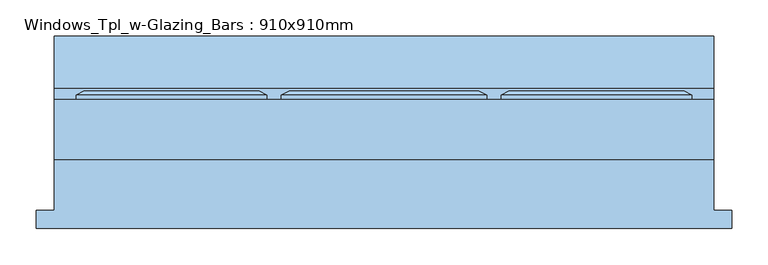
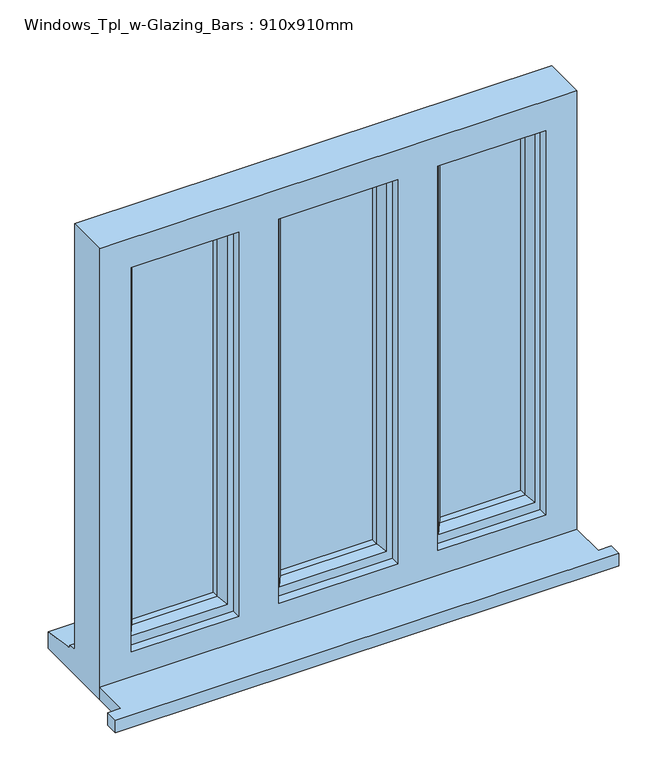
"""IFC4 building model written with IfcOpenShell, lengths in millimetres: window geometry, Windows_Tpl_w-Glazing_Bars : 910x910mm."""

from ifc_helpers import new_model, si_unit, frame, origin, place, context, project, spatial, polyline, outline, extrude, faceted_brep, source, transform, mapped, element, save


def windows_tpl_w_glazing_bars_910x910mm_9d987a72(model_context):
    return source(origin(), model_context, "Body", "SolidModel", [
        extrude(outline(polyline([(-716.6666667, -118.1434322), (-716.6666667, -93.1434322), (-691.6666667, -93.1434322), (-691.6666667, -22.9434322), (218.3333333, -22.9434322), (218.3333333, -93.1434322), (243.3333333, -93.1434322), (243.3333333, -118.1434322), (-716.6666667, -118.1434322)])), frame((0.0, 0.0, 1200.0), z_axis=(0.0, 0.0, 1.0), x_axis=(1.0, 0.0, 0.0)), (0.0, 0.0, 1.0), 25.0),
        faceted_brep([(-75.0, 60.0565678, 2080.0), (-75.0, 65.8300705, 2080.0), (-75.0, 65.8300705, 1253.0), (-75.0, 60.0565678, 1253.0), (-65.0, -4.9434322, 2070.0), (-65.0, 60.0565678, 2070.0), (-65.0, 60.0565678, 1263.0), (-65.0, -4.9434322, 1263.0), (-25.0, 9.5494677, 2030.0), (-35.1480377, -4.9434322, 2040.1480377), (-35.1480377, -4.9434322, 1292.8519623), (-25.0, 9.5494677, 1303.0), (-25.0, 24.0565678, 2030.0), (-25.0, 24.0565678, 1303.0), (-35.0, 48.0565678, 2040.0), (-35.0, 24.0565678, 2040.0), (-35.0, 24.0565678, 1293.0), (-35.0, 48.0565678, 1293.0), (-25.0, 65.8300705, 2030.0), (-25.0, 48.0565678, 2030.0), (-25.0, 48.0565678, 1303.0), (-25.0, 65.8300705, 1303.0), (-42.4457548, 71.6035732, 2047.4457548), (-42.4457548, 71.6035732, 1285.5542452), (-64.2153903, 71.6035732, 2069.2153903), (-64.2153903, 71.6035732, 1263.7846097), (188.3333333, 65.8300705, 1253.0), (188.3333333, 60.0565678, 1253.0), (178.3333333, 60.0565678, 1263.0), (178.3333333, -4.9434322, 1263.0), (148.4813711, -4.9434322, 1292.8519623), (138.3333333, 9.5494677, 1303.0), (138.3333333, 24.0565678, 1303.0), (148.3333333, 24.0565678, 1293.0), (148.3333333, 48.0565678, 1293.0), (138.3333333, 48.0565678, 1303.0), (138.3333333, 65.8300705, 1303.0), (155.7790881, 71.6035732, 1285.5542452), (177.5487236, 71.6035732, 1263.7846097), (188.3333333, 65.8300705, 2080.0), (188.3333333, 60.0565678, 2080.0), (178.3333333, 60.0565678, 2070.0), (178.3333333, -4.9434322, 2070.0), (148.4813711, -4.9434322, 2040.1480377), (138.3333333, 9.5494677, 2030.0), (138.3333333, 24.0565678, 2030.0), (148.3333333, 24.0565678, 2040.0), (148.3333333, 48.0565678, 2040.0), (138.3333333, 48.0565678, 2030.0), (138.3333333, 65.8300705, 2030.0), (155.7790881, 71.6035732, 2047.4457548), (177.5487236, 71.6035732, 2069.2153903)], [[[0, 1, 2, 3]], [[4, 5, 6, 7]], [[8, 9, 10, 11]], [[12, 8, 11, 13]], [[14, 15, 16, 17]], [[18, 19, 20, 21]], [[22, 18, 21, 23]], [[1, 24, 25, 2]], [[3, 2, 26, 27]], [[7, 6, 28, 29]], [[11, 10, 30, 31]], [[13, 11, 31, 32]], [[17, 16, 33, 34]], [[21, 20, 35, 36]], [[23, 21, 36, 37]], [[2, 25, 38, 26]], [[27, 26, 39, 40]], [[29, 28, 41, 42]], [[31, 30, 43, 44]], [[32, 31, 44, 45]], [[34, 33, 46, 47]], [[36, 35, 48, 49]], [[37, 36, 49, 50]], [[26, 38, 51, 39]], [[40, 39, 1, 0]], [[3, 27, 40, 0], [5, 41, 28, 6]], [[42, 41, 5, 4]], [[7, 29, 42, 4], [9, 43, 30, 10]], [[44, 43, 9, 8]], [[45, 44, 8, 12]], [[15, 46, 33, 16], [13, 32, 45, 12]], [[47, 46, 15, 14]], [[17, 34, 47, 14], [19, 48, 35, 20]], [[49, 48, 19, 18]], [[50, 49, 18, 22]], [[24, 51, 38, 25], [23, 37, 50, 22]], [[39, 51, 24, 1]]]),
        extrude(outline(polyline([(148.3333333, 24.0565678), (-35.1480377, 24.0565678), (-35.1480377, 48.0565678), (148.3333333, 48.0565678), (148.3333333, 24.0565678)])), frame((0.0, 0.0, 1293.0), z_axis=(0.0, 0.0, 1.0), x_axis=(1.0, 0.0, 0.0)), (0.0, 0.0, 1.0), 747.0),
        extrude(outline(polyline([(-135.0, 24.0565678), (-338.3333333, 24.0565678), (-338.3333333, 48.0565678), (-135.0, 48.0565678), (-135.0, 24.0565678)])), frame((0.0, 0.0, 1293.0), z_axis=(0.0, 0.0, 1.0), x_axis=(1.0, 0.0, 0.0)), (0.0, 0.0, 1.0), 747.0),
        extrude(outline(polyline([(-438.3333333, 24.0565678), (-621.6666667, 24.0565678), (-621.6666667, 48.0565678), (-438.3333333, 48.0565678), (-438.3333333, 24.0565678)])), frame((0.0, 0.0, 1293.0), z_axis=(0.0, 0.0, 1.0), x_axis=(1.0, 0.0, 0.0)), (0.0, 0.0, 1.0), 747.0),
        faceted_brep([(-398.3333333, 60.0565678, 2080.0), (-398.3333333, 65.8300705, 2080.0), (-661.6666667, 65.8300705, 2080.0), (-661.6666667, 60.0565678, 2080.0), (-408.3333333, -4.9434322, 2070.0), (-408.3333333, 60.0565678, 2070.0), (-651.6666667, 60.0565678, 2070.0), (-651.6666667, -4.9434322, 2070.0), (-448.3333333, 9.5494677, 2030.0), (-438.1852956, -4.9434322, 2040.1480377), (-621.8147044, -4.9434322, 2040.1480377), (-611.6666667, 9.5494677, 2030.0), (-448.3333333, 24.0565678, 2030.0), (-611.6666667, 24.0565678, 2030.0), (-438.3333333, 48.0565678, 2040.0), (-438.3333333, 24.0565678, 2040.0), (-621.6666667, 24.0565678, 2040.0), (-621.6666667, 48.0565678, 2040.0), (-448.3333333, 65.8300705, 2030.0), (-448.3333333, 48.0565678, 2030.0), (-611.6666667, 48.0565678, 2030.0), (-611.6666667, 65.8300705, 2030.0), (-430.8875785, 71.6035732, 2047.4457548), (-629.1124215, 71.6035732, 2047.4457548), (-409.117943, 71.6035732, 2069.2153903), (-650.882057, 71.6035732, 2069.2153903), (-661.6666667, 65.8300705, 1253.0), (-661.6666667, 60.0565678, 1253.0), (-651.6666667, 60.0565678, 1263.0), (-651.6666667, -4.9434322, 1263.0), (-621.8147044, -4.9434322, 1292.8519623), (-611.6666667, 9.5494677, 1303.0), (-611.6666667, 24.0565678, 1303.0), (-621.6666667, 24.0565678, 1293.0), (-621.6666667, 48.0565678, 1293.0), (-611.6666667, 48.0565678, 1303.0), (-611.6666667, 65.8300705, 1303.0), (-629.1124215, 71.6035732, 1285.5542452), (-650.882057, 71.6035732, 1263.7846097), (-398.3333333, 65.8300705, 1253.0), (-398.3333333, 60.0565678, 1253.0), (-408.3333333, 60.0565678, 1263.0), (-408.3333333, -4.9434322, 1263.0), (-438.1852956, -4.9434322, 1292.8519623), (-448.3333333, 9.5494677, 1303.0), (-448.3333333, 24.0565678, 1303.0), (-438.3333333, 24.0565678, 1293.0), (-438.3333333, 48.0565678, 1293.0), (-448.3333333, 48.0565678, 1303.0), (-448.3333333, 65.8300705, 1303.0), (-430.8875785, 71.6035732, 1285.5542452), (-409.117943, 71.6035732, 1263.7846097)], [[[0, 1, 2, 3]], [[4, 5, 6, 7]], [[8, 9, 10, 11]], [[12, 8, 11, 13]], [[14, 15, 16, 17]], [[18, 19, 20, 21]], [[22, 18, 21, 23]], [[1, 24, 25, 2]], [[3, 2, 26, 27]], [[7, 6, 28, 29]], [[11, 10, 30, 31]], [[13, 11, 31, 32]], [[17, 16, 33, 34]], [[21, 20, 35, 36]], [[23, 21, 36, 37]], [[2, 25, 38, 26]], [[27, 26, 39, 40]], [[0, 3, 27, 40], [41, 28, 6, 5]], [[29, 28, 41, 42]], [[4, 7, 29, 42], [43, 30, 10, 9]], [[31, 30, 43, 44]], [[32, 31, 44, 45]], [[46, 33, 16, 15], [12, 13, 32, 45]], [[34, 33, 46, 47]], [[14, 17, 34, 47], [48, 35, 20, 19]], [[36, 35, 48, 49]], [[37, 36, 49, 50]], [[51, 38, 25, 24], [22, 23, 37, 50]], [[26, 38, 51, 39]], [[40, 39, 1, 0]], [[42, 41, 5, 4]], [[44, 43, 9, 8]], [[45, 44, 8, 12]], [[47, 46, 15, 14]], [[49, 48, 19, 18]], [[50, 49, 18, 22]], [[39, 51, 24, 1]]]),
        extrude(outline(polyline([(-35.0, 40.0565678), (148.3333333, 40.0565678), (148.3333333, 32.0565678), (-35.0, 32.0565678), (-35.0, 40.0565678)])), frame((0.0, 0.0, 1656.5), z_axis=(0.0, 0.0, 1.0), x_axis=(1.0, 0.0, 0.0)), (0.0, 0.0, 1.0), 20.0),
        extrude(outline(polyline([(-621.6666667, 40.0565678), (-438.3333333, 40.0565678), (-438.3333333, 32.0565678), (-621.6666667, 32.0565678), (-621.6666667, 40.0565678)])), frame((0.0, 0.0, 1656.5), z_axis=(0.0, 0.0, 1.0), x_axis=(1.0, 0.0, 0.0)), (0.0, 0.0, 1.0), 20.0),
        extrude(outline(polyline([(-35.0, 40.0565678), (148.3333333, 40.0565678), (148.3333333, 32.0565678), (-35.0, 32.0565678), (-35.0, 40.0565678)])), frame((0.0, 0.0, 1838.25), z_axis=(0.0, 0.0, 1.0), x_axis=(1.0, 0.0, 0.0)), (0.0, 0.0, 1.0), 20.0),
        extrude(outline(polyline([(-35.0, 40.0565678), (148.3333333, 40.0565678), (148.3333333, 32.0565678), (-35.0, 32.0565678), (-35.0, 40.0565678)])), frame((0.0, 0.0, 1474.75), z_axis=(0.0, 0.0, 1.0), x_axis=(1.0, 0.0, 0.0)), (0.0, 0.0, 1.0), 20.0),
        extrude(outline(polyline([(-621.6666667, 40.0565678), (-438.3333333, 40.0565678), (-438.3333333, 32.0565678), (-621.6666667, 32.0565678), (-621.6666667, 40.0565678)])), frame((0.0, 0.0, 1838.25), z_axis=(0.0, 0.0, 1.0), x_axis=(1.0, 0.0, 0.0)), (0.0, 0.0, 1.0), 20.0),
        extrude(outline(polyline([(-621.6666667, 40.0565678), (-438.3333333, 40.0565678), (-438.3333333, 32.0565678), (-621.6666667, 32.0565678), (-621.6666667, 40.0565678)])), frame((0.0, 0.0, 1474.75), z_axis=(0.0, 0.0, 1.0), x_axis=(1.0, 0.0, 0.0)), (0.0, 0.0, 1.0), 20.0),
        extrude(outline(polyline([(-338.3333333, 40.0565678), (-135.0, 40.0565678), (-135.0, 32.0565678), (-338.3333333, 32.0565678), (-338.3333333, 40.0565678)])), frame((0.0, 0.0, 1656.5), z_axis=(0.0, 0.0, 1.0), x_axis=(1.0, 0.0, 0.0)), (0.0, 0.0, 1.0), 20.0),
        extrude(outline(polyline([(-338.3333333, 40.0565678), (-135.0, 40.0565678), (-135.0, 32.0565678), (-338.3333333, 32.0565678), (-338.3333333, 40.0565678)])), frame((0.0, 0.0, 1838.25), z_axis=(0.0, 0.0, 1.0), x_axis=(1.0, 0.0, 0.0)), (0.0, 0.0, 1.0), 20.0),
        extrude(outline(polyline([(-338.3333333, 40.0565678), (-135.0, 40.0565678), (-135.0, 32.0565678), (-338.3333333, 32.0565678), (-338.3333333, 40.0565678)])), frame((0.0, 0.0, 1474.75), z_axis=(0.0, 0.0, 1.0), x_axis=(1.0, 0.0, 0.0)), (0.0, 0.0, 1.0), 20.0),
        faceted_brep([(218.3333333, -22.9434322, 2110.0), (-691.6666667, -22.9434322, 2110.0), (-691.6666667, -22.9434322, 1200.0), (218.3333333, -22.9434322, 1200.0), (158.3333333, -22.9434322, 2050.0), (158.3333333, -22.9434322, 1275.0), (-47.0, -22.9434322, 1275.0), (-47.0, -22.9434322, 2050.0), (-123.0, -22.9434322, 2050.0), (-123.0, -22.9434322, 1275.0), (-350.3333333, -22.9434322, 1275.0), (-350.3333333, -22.9434322, 2050.0), (-426.3333333, -22.9434322, 2050.0), (-426.3333333, -22.9434322, 1275.0), (-631.6666667, -22.9434322, 1275.0), (-631.6666667, -22.9434322, 2050.0), (-691.6666667, 60.0565678, 2110.0), (-691.6666667, 60.0565678, 1251.0), (-691.6666667, 75.0565678, 1249.68767), (-691.6666667, 75.0565678, 1244.7449676), (-691.6666667, 147.5565678, 1233.8088847), (-691.6666667, 147.5565678, 1200.0), (218.3333333, 60.0565678, 2110.0), (218.3333333, 60.0565678, 1251.0), (-651.6666667, 60.0565678, 2070.0), (-651.6666667, 60.0565678, 1263.0), (-408.3333333, 60.0565678, 1263.0), (-408.3333333, 60.0565678, 2070.0), (-368.3333333, 60.0565678, 2070.0), (-368.3333333, 60.0565678, 1263.0), (-105.0, 60.0565678, 1263.0), (-105.0, 60.0565678, 2070.0), (-65.0, 60.0565678, 2070.0), (-65.0, 60.0565678, 1263.0), (178.3333333, 60.0565678, 1263.0), (178.3333333, 60.0565678, 2070.0), (-651.6666667, -4.9434322, 2070.0), (-651.6666667, -4.9434322, 1263.0), (-368.3333333, -4.9434322, 2070.0), (-105.0, -4.9434322, 2070.0), (-105.0, -4.9434322, 1263.0), (-368.3333333, -4.9434322, 1263.0), (-123.0, -4.9434322, 2050.0), (-350.3333333, -4.9434322, 2050.0), (-350.3333333, -4.9434322, 1275.0), (-123.0, -4.9434322, 1275.0), (-65.0, -4.9434322, 2070.0), (178.3333333, -4.9434322, 2070.0), (178.3333333, -4.9434322, 1263.0), (-65.0, -4.9434322, 1263.0), (158.3333333, -4.9434322, 2050.0), (-47.0, -4.9434322, 2050.0), (-47.0, -4.9434322, 1275.0), (158.3333333, -4.9434322, 1275.0), (-408.3333333, -4.9434322, 2070.0), (-408.3333333, -4.9434322, 1263.0), (-426.3333333, -4.9434322, 2050.0), (-631.6666667, -4.9434322, 2050.0), (-631.6666667, -4.9434322, 1275.0), (-426.3333333, -4.9434322, 1275.0), (218.3333333, 147.5565678, 1200.0), (218.3333333, 147.5565678, 1233.8088847), (218.3333333, 75.0565678, 1244.7449676), (218.3333333, 75.0565678, 1249.68767)], [[[0, 1, 2, 3], [4, 5, 6, 7], [8, 9, 10, 11], [12, 13, 14, 15]], [[2, 1, 16, 17, 18, 19, 20, 21]], [[17, 16, 22, 23], [24, 25, 26, 27], [28, 29, 30, 31], [32, 33, 34, 35]], [[25, 24, 36, 37]], [[38, 39, 40, 41], [42, 43, 44, 45]], [[46, 47, 48, 49], [50, 51, 52, 53]], [[36, 54, 55, 37], [56, 57, 58, 59]], [[57, 15, 14, 58]], [[1, 0, 22, 16]], [[36, 24, 27, 54]], [[35, 47, 46, 32]], [[38, 28, 31, 39]], [[15, 57, 56, 12]], [[50, 4, 7, 51]], [[11, 43, 42, 8]], [[23, 22, 0, 3, 60, 61, 62, 63]], [[35, 34, 48, 47]], [[4, 50, 53, 5]], [[43, 11, 10, 44]], [[12, 56, 59, 13]], [[27, 26, 55, 54]], [[29, 28, 38, 41]], [[31, 30, 40, 39]], [[33, 32, 46, 49]], [[51, 7, 6, 52]], [[8, 42, 45, 9]], [[60, 3, 2, 21]], [[61, 60, 21, 20]], [[62, 61, 20, 19]], [[63, 62, 19, 18]], [[23, 63, 18, 17]], [[26, 25, 37, 55]], [[34, 33, 49, 48]], [[41, 40, 30, 29]], [[6, 5, 53, 52]], [[45, 44, 10, 9]], [[59, 58, 14, 13]]]),
        faceted_brep([(-378.3333333, 60.0565678, 2080.0), (-378.3333333, 65.8300705, 2080.0), (-378.3333333, 65.8300705, 1253.0), (-378.3333333, 60.0565678, 1253.0), (-368.3333333, -4.9434322, 2070.0), (-368.3333333, 60.0565678, 2070.0), (-368.3333333, 60.0565678, 1263.0), (-368.3333333, -4.9434322, 1263.0), (-328.3333333, 9.5494677, 2030.0), (-338.4813711, -4.9434322, 2040.1480377), (-338.4813711, -4.9434322, 1292.8519623), (-328.3333333, 9.5494677, 1303.0), (-328.3333333, 24.0565678, 2030.0), (-328.3333333, 24.0565678, 1303.0), (-338.3333333, 48.0565678, 2040.0), (-338.3333333, 24.0565678, 2040.0), (-338.3333333, 24.0565678, 1293.0), (-338.3333333, 48.0565678, 1293.0), (-328.3333333, 65.8300705, 2030.0), (-328.3333333, 48.0565678, 2030.0), (-328.3333333, 48.0565678, 1303.0), (-328.3333333, 65.8300705, 1303.0), (-345.7790881, 71.6035732, 2047.4457548), (-345.7790881, 71.6035732, 1285.5542452), (-367.5487236, 71.6035732, 2069.2153903), (-367.5487236, 71.6035732, 1263.7846097), (-95.0, 65.8300705, 1253.0), (-95.0, 60.0565678, 1253.0), (-105.0, 60.0565678, 1263.0), (-105.0, -4.9434322, 1263.0), (-134.8519623, -4.9434322, 1292.8519623), (-145.0, 9.5494677, 1303.0), (-145.0, 24.0565678, 1303.0), (-135.0, 24.0565678, 1293.0), (-135.0, 48.0565678, 1293.0), (-145.0, 48.0565678, 1303.0), (-145.0, 65.8300705, 1303.0), (-127.5542452, 71.6035732, 1285.5542452), (-105.7846097, 71.6035732, 1263.7846097), (-95.0, 65.8300705, 2080.0), (-95.0, 60.0565678, 2080.0), (-105.0, 60.0565678, 2070.0), (-105.0, -4.9434322, 2070.0), (-134.8519623, -4.9434322, 2040.1480377), (-145.0, 9.5494677, 2030.0), (-145.0, 24.0565678, 2030.0), (-135.0, 24.0565678, 2040.0), (-135.0, 48.0565678, 2040.0), (-145.0, 48.0565678, 2030.0), (-145.0, 65.8300705, 2030.0), (-127.5542452, 71.6035732, 2047.4457548), (-105.7846097, 71.6035732, 2069.2153903)], [[[0, 1, 2, 3]], [[4, 5, 6, 7]], [[8, 9, 10, 11]], [[12, 8, 11, 13]], [[14, 15, 16, 17]], [[18, 19, 20, 21]], [[22, 18, 21, 23]], [[1, 24, 25, 2]], [[3, 2, 26, 27]], [[7, 6, 28, 29]], [[11, 10, 30, 31]], [[13, 11, 31, 32]], [[17, 16, 33, 34]], [[21, 20, 35, 36]], [[23, 21, 36, 37]], [[2, 25, 38, 26]], [[27, 26, 39, 40]], [[29, 28, 41, 42]], [[31, 30, 43, 44]], [[32, 31, 44, 45]], [[34, 33, 46, 47]], [[36, 35, 48, 49]], [[37, 36, 49, 50]], [[26, 38, 51, 39]], [[40, 39, 1, 0]], [[3, 27, 40, 0], [5, 41, 28, 6]], [[42, 41, 5, 4]], [[7, 29, 42, 4], [9, 43, 30, 10]], [[44, 43, 9, 8]], [[45, 44, 8, 12]], [[15, 46, 33, 16], [13, 32, 45, 12]], [[47, 46, 15, 14]], [[17, 34, 47, 14], [19, 48, 35, 20]], [[49, 48, 19, 18]], [[50, 49, 18, 22]], [[24, 51, 38, 25], [23, 37, 50, 22]], [[39, 51, 24, 1]]]),
    ])


if __name__ == "__main__":
    model = new_model("IFC4")
    model_context = context("Model", 3, world=origin())
    ifc_project = project(units=[si_unit("LENGTHUNIT", "METRE", prefix="MILLI")], contexts=[model_context])
    site = spatial("IfcSite", under=ifc_project)
    building = spatial("IfcBuilding", under=site)
    placement = place(None, origin())
    windows_tpl_w_glazing_bars_910x910mm_shape = windows_tpl_w_glazing_bars_910x910mm_9d987a72(model_context)
    element("IfcWindow", 1, ObjectType="Windows_Tpl_w-Glazing_Bars : 910x910mm", at=placement, inside=building, context=model_context, shape_type="MappedRepresentation", body=[
        mapped(windows_tpl_w_glazing_bars_910x910mm_shape, transform((0.0, 0.0, 0.0), x_axis=(1.0, 0.0, 0.0), y_axis=(0.0, 1.0, 0.0), z_axis=(0.0, 0.0, 1.0))),
    ])
    save(model, "model.ifc")

# Revit data of these elements
# Type "Windows_Tpl_w-Glazing_Bars : 910x910mm"
#   Type Mark = "18"
#   Operation = "TriplePanelVertical"
#   Construction Type Id = "GSP4R"
#   Manufacturer = "Revit"
#   Keynote = "L10"
#   Analytic Construction = "1/8 in Pilkington single glazing"
#   Length 1 = 0' - 0.94488"
#   Wrap Layers (Ext) from Ext = 0' - 4.03543"
#   Wrap Layers (Int) from Ext = 0' - 6.98819"
#   Window Board Projection = 0' - 0.98425"
#   Window Board Extension = 0' - 0.98425"
#   Visual Light Transmittance = 0.9
#   Solar Heat Gain Coefficient = 0.78
#   Rough Width = 2' - 11.82677"
#   Rough Height = 2' - 11.82677"
#   Height = 2' - 11.82677"
#   Width = 2' - 11.82677"
#   Heat Transfer Coefficient (U) = 0.6496 BTU/(h·ft²·°F)
#   Glazing Thickness = 0' - 0.94488"
#   Glazing Bar Thickness = 0' - 0.7874"
#   FrameOffset - External = 0' - 1.9685"
#   Frame Depth = 0' - 2.55906"
#   Default Head Height = 6' - 11.07087"
#   Cill Depth = 0' - 3.44488"
#   Cavity Closer Width = 0' - 1.9685"
#   Cavity Closer Offset from Ext = 0' - 4.03543"
#   Cavity Closer Depth = 0' - 3.34646"
#   Vis - Glazing Bars = yes
#   Vis - Cavity Closers = yes
#   Define Thermal Properties by = 1
#   Material Trim = Window Frame
#   Material Glazing Bars = Window Frame
#   Material Glass = Glass
#   Material Frame = Window Frame
#   Wall Closure = (empty or 0)
# Element 1 (IfcWindow, "Windows_Tpl_w-Glazing_Bars : 910x910mm")
#   Materials on its faces: "Window Frame", "Glass"
# Materials
#   "Window Frame": colour RGB 249 249 249, transparency 0
#   "Glass": class "Glass", colour RGB 0 128 192, transparency 0.75, Description = "Soda Lime Glass", Cost = 0
